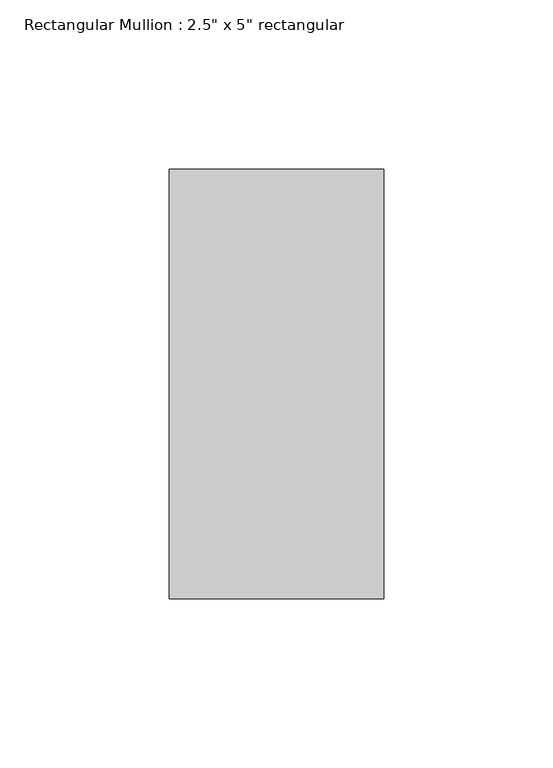
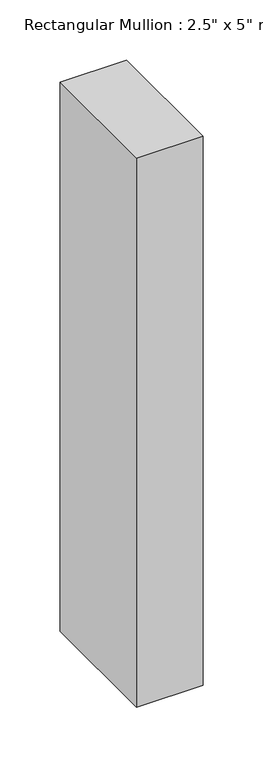
"""IFC4 building model written with IfcOpenShell, lengths in millimetres: member geometry."""

from ifc_helpers import new_model, si_unit, frame, origin, place, context, project, spatial, polyline, outline, extrude, source, transform, mapped, element, save


def member_b26d3c89(model_context):
    return source(origin(), model_context, "Body", "SweptSolid", [
        extrude(outline(polyline([(0.0, 63.5), (0.0, -63.5), (-63.5, -63.5), (-63.5, 63.5), (0.0, 63.5)])), frame((0.0, 0.0, -556.6833334), z_axis=(0.0, 0.0, 1.0), x_axis=(1.0, 0.0, 0.0)), (0.0, 0.0, 1.0), 556.6833334),
    ])


if __name__ == "__main__":
    model = new_model("IFC4")
    model_context = context("Model", 3, world=origin())
    ifc_project = project(units=[si_unit("LENGTHUNIT", "METRE", prefix="MILLI")], contexts=[model_context])
    site = spatial("IfcSite", under=ifc_project)
    building = spatial("IfcBuilding", under=site)
    placement = place(None, origin())
    member_shape = member_b26d3c89(model_context)
    element("IfcMember", 1, ObjectType="Rectangular Mullion : 2.5\" x 5\" rectangular", at=placement, inside=building, context=model_context, shape_type="MappedRepresentation", body=[
        mapped(member_shape, transform((0.0, 0.0, 0.0), x_axis=(1.0, 0.0, 0.0), y_axis=(0.0, 1.0, 0.0), z_axis=(0.0, 0.0, 1.0))),
    ])
    save(model, "model.ifc")

# Revit data of these elements
# Type "Rectangular Mullion : 2.5\" x 5\" rectangular"
#   built-in parameter 1007304 = 0.416667 (stored number, unit not read)
#   built-in parameter 1007301 = 0.104167 (stored number, unit not read)
#   built-in parameter 1007300 = 0.104167 (stored number, unit not read)
# Element 1 (IfcMember, "Rectangular Mullion : 2.5\" x 5\" rectangular")
#   Materials on its faces: "Aluminum"
# Materials
#   "Aluminum": class "Metal", colour RGB 247 247 247, transparency 0, Description = "Aluminum 6061", Cost = 0
